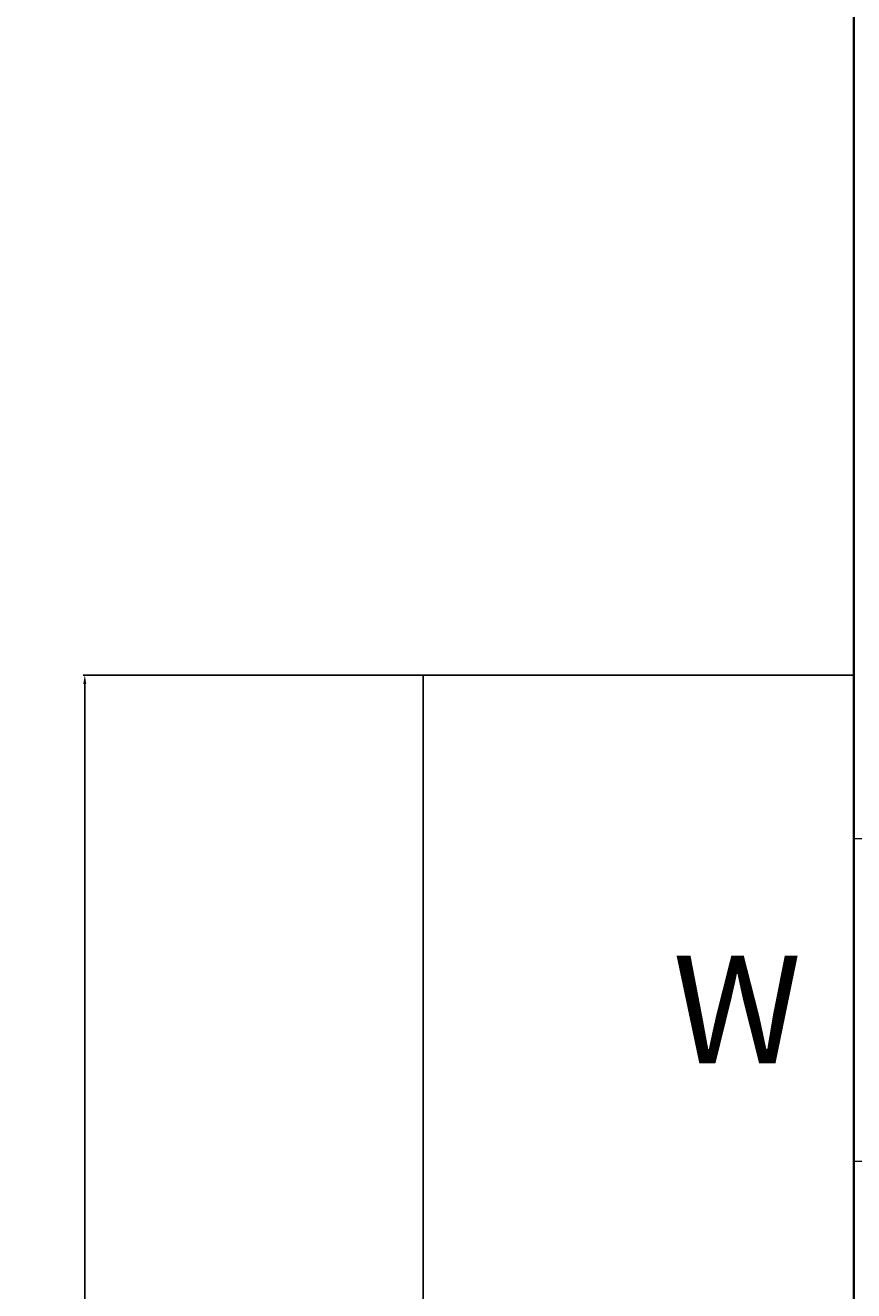
# Model space of a CAD drawing. Units: inches. Extents: x -304 to 580, y 363 to 1149.
# Tile 5 of 11: x -115 to -23, y 653 to 794. Entities that reach past the tile are written whole.
import ezdxf

# ---------------------------------------------------------------- set-up
doc = ezdxf.new("R2010")
doc.units = ezdxf.units.IN
doc.header["$MEASUREMENT"] = 0
for name, color, linetype, lineweight in [('A-ANNO-DIMS', 2, 'Continuous', 13), ('A-ANNO-IDEN', 7, 'Continuous', 18), ('A-FLOR-OTLN', 2, 'Continuous', 25), ('A-GLAZ', 4, 'Continuous', 18), ('A-WALL', 40, 'Continuous', 35)]:
    doc.layers.add(name, color=color, linetype=linetype, lineweight=lineweight)
doc.styles.get("Standard").update_dxf_attribs({"font": 'arial.ttf'})
doc.dimstyles.get("Standard").update_dxf_attribs({"dimtxt": 1, "dimasz": 1, "dimexe": 0.18, "dimexo": 0.0625, "dimgap": 0.09, "dimtad": 0, "dimtih": 1, "dimtoh": 1, "dimdec": 0, "dimzin": 0, "dimdsep": 46, "dimlunit": 3, "dimtxsty": 'Standard', "dimcen": 0.09, "dimadec": 0, "dimazin": 0, "dimtfac": 1, "dimtdec": 0, "dimtofl": 0, "dimtmove": 0, "dimatfit": 3, "dimfxl": 1, "dimtolj": 1, "dimtzin": 0, "dimarcsym": 0})

# ---------------------------------------------------------------- blocks, each defined once
blk = doc.blocks.new('*D1')
at = {"layer": 'A-ANNO-DIMS', "color": 0, "lineweight": -2, "transparency": 16777216}
for p, q in [((-22.63, 1004.95), (-237.62, 1004.95)), ((-237.44, 1003.95), (-237.44, 721.93)), ((-237.44, 402.95), (-237.44, 684.96)), ((-22.63, 401.95), (-237.62, 401.95))]:
    blk.add_line(p, q, dxfattribs=at)
at = {"layer": 'A-ANNO-DIMS', "color": 0, "transparency": 16777216}
for points in [[(-237.61, 1003.95), (-237.28, 1003.95), (-237.44, 1004.95)], [(-237.61, 402.95), (-237.28, 402.95), (-237.44, 401.95)]]:
    blk.add_solid(points, dxfattribs=at)
at = {"layer": 'Defpoints', "color": 0, "transparency": 16777216}
for p in [(-22.57, 1004.95), (-237.44, 401.95), (-22.57, 401.95)]:
    blk.add_point(p, dxfattribs=at)
at = {"layer": 'A-ANNO-DIMS', "color": 0, "transparency": 16777216, "insert": (-237.44, 703.45), "char_height": 1, "attachment_point": 5}
blk.add_mtext('\\A1;{\\H36x;50\'-3"}', dxfattribs=at)
blk = doc.blocks.new('WIN-36IN')
for p, q in [((0, 6.5), (36, 6.5)), ((0, 4.5), (36, 4.5)), ((0, 2.5), (36, 2.5))]:
    blk.add_line(p, q)
blk.add_lwpolyline([(0, 0), (0, 9), (36, 9), (36, 0)], close=True)
blk = doc.blocks.new('*D30')
at = {"layer": 'A-ANNO-DIMS', "color": 0, "lineweight": -2, "transparency": 16777216}
for p, q in [((-70.63, 721.98), (-108.5, 721.98)), ((-108.32, 720.98), (-108.32, 562.56)), ((-108.32, 402.95), (-108.32, 561.36)), ((-70.63, 401.95), (-108.5, 401.95))]:
    blk.add_line(p, q, dxfattribs=at)
at = {"layer": 'A-ANNO-DIMS', "color": 0, "transparency": 16777216}
for points in [[(-108.49, 720.98), (-108.15, 720.98), (-108.32, 721.98)], [(-108.49, 402.95), (-108.15, 402.95), (-108.32, 401.95)]]:
    blk.add_solid(points, dxfattribs=at)
at = {"layer": 'Defpoints', "color": 0, "transparency": 16777216}
for p in [(-108.32, 721.98), (-70.57, 721.98), (-70.57, 401.95)]:
    blk.add_point(p, dxfattribs=at)
at = {"layer": 'A-ANNO-DIMS', "color": 0, "transparency": 16777216, "insert": (-108.32, 561.96), "char_height": 1, "attachment_point": 5}
blk.add_mtext('\\A1;26\'-8"', dxfattribs=at)

msp = doc.modelspace()

# ---------------------------------------------------------------- linework, layer by layer
at = {"layer": 'A-FLOR-OTLN'}
for p, q in [((-22.57, 721.98), (-70.57, 721.98)), ((-70.57, 721.98), (-70.57, 401.95))]:
    msp.add_line(p, q, dxfattribs=at)
at = {"layer": 'A-WALL'}
msp.add_line((-22.57, 516.51), (-22.57, 1004.95), dxfattribs=at)

# ---------------------------------------------------------------- block references
at = {"layer": 'A-GLAZ', "rotation": 270.0000000000002}
msp.add_blockref('WIN-36IN', (-22.57, 703.75), dxfattribs=at)

# ---------------------------------------------------------------- texts
at = {"layer": 'A-ANNO-IDEN', "insert": (-42.75, 690.69), "char_height": 12, "attachment_point": 1}
msp.add_mtext_dynamic_manual_height_columns('W', width=41.6501, gutter_width=1, heights=[0], dxfattribs=at)

# ---------------------------------------------------------------- dimensions: what is measured, and where the dimension line sits
at = {"layer": 'A-ANNO-DIMS'}
dim = msp.add_linear_dim(base=(-237.44, 401.95), p1=(-22.57, 1004.95), p2=(-22.57, 401.95), angle=90, text='{\\H36x;<>}', dimstyle='Standard', override={"dimclrd": 0, "dimclre": 0, "dimclrt": 0}, dxfattribs=at)
dim.commit()
dim.dimension.update_dxf_attribs({"geometry": '*D1', "text_midpoint": (-237.44, 703.45)})
dim = msp.add_linear_dim(base=(-108.32, 721.98), p1=(-70.57, 401.95), p2=(-70.57, 721.98), angle=90, dimstyle='Standard', override={"dimdec": 1, "dimlfac": 1, "dimrnd": 0, "dimzin": 1, "dimdsep": 46, "dimlunit": 4, "dimfrac": 2}, dxfattribs=at)
dim.commit()
dim.dimension.update_dxf_attribs({"geometry": '*D30', "text_midpoint": (-108.32, 561.96)})

doc.saveas('drawing.dxf')
